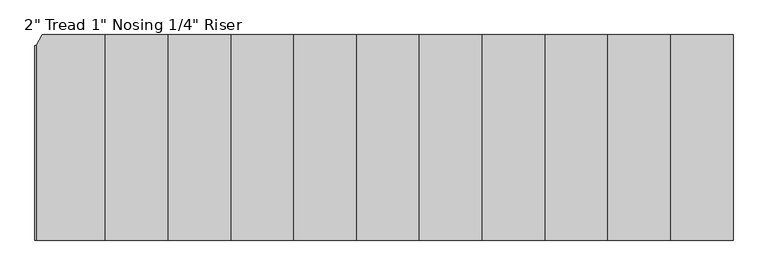
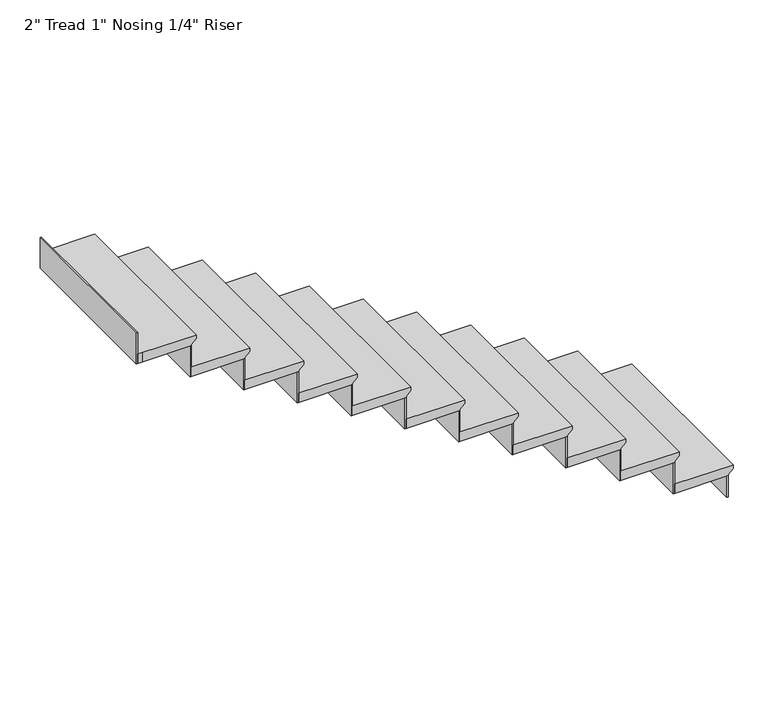
"""IFC4 building model written with IfcOpenShell, lengths in millimetres: stair flight geometry."""

from ifc_helpers import new_model, si_unit, origin, place, context, project, spatial, faceted_brep, source, transform, mapped, element, save


def stair_flight_13c2be00(model_context):
    return source(origin(), model_context, "Body", "Brep", [
        faceted_brep([(-10702.6822797, 5301.3500793, 150.2833333), (-10702.6822797, 5301.3500793, 169.3333333), (-10702.6822797, 4386.9500793, 169.3333333), (-10702.6822797, 4386.9500793, 150.2833333), (-10728.0822797, 5301.3500793, 124.8833333), (-10728.0822797, 4386.9500793, 124.8833333), (-11007.4822797, 5301.3500793, 169.3333333), (-11007.4822797, 4386.9500793, 169.3333333), (-10728.0822797, 4386.9500793, 118.5333333), (-11007.4822797, 4386.9500793, 118.5333333), (-11007.4822797, 5301.3500793, 118.5333333), (-10728.0822797, 5301.3500793, 118.5333333)], [[[0, 1, 2, 3]], [[4, 0, 3, 5]], [[2, 1, 6, 7]], [[8, 9, 10, 11]], [[2, 7, 9, 8, 5, 3]], [[8, 11, 4, 5]], [[6, 1, 0, 4, 11, 10]], [[7, 6, 10, 9]]]),
        faceted_brep([(-10728.0822797, 5301.3500793, 118.5333333), (-10728.0822797, 5301.3500793, 0.0), (-10734.4322797, 5301.3500793, 0.0), (-10734.4322797, 5301.3500793, 118.5333333), (-10728.0822797, 4386.9500793, 118.5333333), (-10734.4322797, 4386.9500793, 118.5333333), (-10734.4322797, 4386.9500793, 0.0), (-10728.0822797, 4386.9500793, 0.0)], [[[0, 1, 2, 3]], [[4, 5, 6, 7]], [[1, 0, 4, 7]], [[2, 1, 7, 6]], [[3, 2, 6, 5]], [[0, 3, 5, 4]]]),
        faceted_brep([(-11007.4822797, 5301.3500793, 287.8666667), (-11007.4822797, 5301.3500793, 118.5333333), (-11013.8322797, 5301.3500793, 118.5333333), (-11013.8322797, 5301.3500793, 287.8666667), (-11007.4822797, 4386.9500793, 287.8666667), (-11013.8322797, 4386.9500793, 287.8666667), (-11013.8322797, 4386.9500793, 118.5333333), (-11007.4822797, 4386.9500793, 118.5333333)], [[[0, 1, 2, 3]], [[4, 5, 6, 7]], [[1, 0, 4, 7]], [[2, 1, 7, 6]], [[3, 2, 6, 5]], [[0, 3, 5, 4]]]),
        faceted_brep([(-10982.0822797, 4386.9500793, 338.6666667), (-10982.0822797, 5301.3500793, 338.6666667), (-11286.8822797, 5301.3500793, 338.6666667), (-11286.8822797, 4386.9500793, 338.6666667), (-11007.4822797, 4386.9500793, 287.8666667), (-11286.8822797, 4386.9500793, 287.8666667), (-11286.8822797, 5301.3500793, 287.8666667), (-11007.4822797, 5301.3500793, 287.8666667), (-11007.4822797, 4386.9500793, 294.2166667), (-10982.0822797, 4386.9500793, 319.6166667), (-11007.4822797, 5301.3500793, 294.2166667), (-10982.0822797, 5301.3500793, 319.6166667)], [[[0, 1, 2, 3]], [[4, 5, 6, 7]], [[0, 3, 5, 4, 8, 9]], [[4, 7, 10, 8]], [[2, 1, 11, 10, 7, 6]], [[3, 2, 6, 5]], [[11, 1, 0, 9]], [[10, 11, 9, 8]]]),
        faceted_brep([(-11286.8822797, 5301.3500793, 457.2), (-11286.8822797, 5301.3500793, 287.8666667), (-11293.2322797, 5301.3500793, 287.8666667), (-11293.2322797, 5301.3500793, 457.2), (-11286.8822797, 4386.9500793, 457.2), (-11293.2322797, 4386.9500793, 457.2), (-11293.2322797, 4386.9500793, 287.8666667), (-11286.8822797, 4386.9500793, 287.8666667)], [[[0, 1, 2, 3]], [[4, 5, 6, 7]], [[1, 0, 4, 7]], [[2, 1, 7, 6]], [[3, 2, 6, 5]], [[0, 3, 5, 4]]]),
        faceted_brep([(-11261.4822797, 4386.9500793, 508.0), (-11261.4822797, 5301.3500793, 508.0), (-11566.2822797, 5301.3500793, 508.0), (-11566.2822797, 4386.9500793, 508.0), (-11286.8822797, 4386.9500793, 457.2), (-11566.2822797, 4386.9500793, 457.2), (-11566.2822797, 5301.3500793, 457.2), (-11286.8822797, 5301.3500793, 457.2), (-11286.8822797, 4386.9500793, 463.55), (-11261.4822797, 4386.9500793, 488.95), (-11286.8822797, 5301.3500793, 463.55), (-11261.4822797, 5301.3500793, 488.95)], [[[0, 1, 2, 3]], [[4, 5, 6, 7]], [[0, 3, 5, 4, 8, 9]], [[4, 7, 10, 8]], [[2, 1, 11, 10, 7, 6]], [[3, 2, 6, 5]], [[11, 1, 0, 9]], [[10, 11, 9, 8]]]),
        faceted_brep([(-11566.2822797, 5301.3500793, 626.5333333), (-11566.2822797, 5301.3500793, 457.2), (-11572.6322797, 5301.3500793, 457.2), (-11572.6322797, 5301.3500793, 626.5333333), (-11566.2822797, 4386.9500793, 626.5333333), (-11572.6322797, 4386.9500793, 626.5333333), (-11572.6322797, 4386.9500793, 457.2), (-11566.2822797, 4386.9500793, 457.2)], [[[0, 1, 2, 3]], [[4, 5, 6, 7]], [[1, 0, 4, 7]], [[2, 1, 7, 6]], [[3, 2, 6, 5]], [[0, 3, 5, 4]]]),
        faceted_brep([(-11540.8822797, 4386.9500793, 677.3333333), (-11540.8822797, 5301.3500793, 677.3333333), (-11845.6822797, 5301.3500793, 677.3333333), (-11845.6822797, 4386.9500793, 677.3333333), (-11566.2822797, 4386.9500793, 626.5333333), (-11845.6822797, 4386.9500793, 626.5333333), (-11845.6822797, 5301.3500793, 626.5333333), (-11566.2822797, 5301.3500793, 626.5333333), (-11566.2822797, 4386.9500793, 632.8833333), (-11540.8822797, 4386.9500793, 658.2833333), (-11566.2822797, 5301.3500793, 632.8833333), (-11540.8822797, 5301.3500793, 658.2833333)], [[[0, 1, 2, 3]], [[4, 5, 6, 7]], [[0, 3, 5, 4, 8, 9]], [[4, 7, 10, 8]], [[2, 1, 11, 10, 7, 6]], [[3, 2, 6, 5]], [[11, 1, 0, 9]], [[10, 11, 9, 8]]]),
        faceted_brep([(-11845.6822797, 5301.3500793, 795.8666667), (-11845.6822797, 5301.3500793, 626.5333333), (-11852.0322797, 5301.3500793, 626.5333333), (-11852.0322797, 5301.3500793, 795.8666667), (-11845.6822797, 4386.9500793, 795.8666667), (-11852.0322797, 4386.9500793, 795.8666667), (-11852.0322797, 4386.9500793, 626.5333333), (-11845.6822797, 4386.9500793, 626.5333333)], [[[0, 1, 2, 3]], [[4, 5, 6, 7]], [[1, 0, 4, 7]], [[2, 1, 7, 6]], [[3, 2, 6, 5]], [[0, 3, 5, 4]]]),
        faceted_brep([(-11820.2822797, 4386.9500793, 846.6666667), (-11820.2822797, 5301.3500793, 846.6666667), (-12125.0822797, 5301.3500793, 846.6666667), (-12125.0822797, 4386.9500793, 846.6666667), (-11845.6822797, 4386.9500793, 795.8666667), (-12125.0822797, 4386.9500793, 795.8666667), (-12125.0822797, 5301.3500793, 795.8666667), (-11845.6822797, 5301.3500793, 795.8666667), (-11845.6822797, 4386.9500793, 802.2166667), (-11820.2822797, 4386.9500793, 827.6166667), (-11845.6822797, 5301.3500793, 802.2166667), (-11820.2822797, 5301.3500793, 827.6166667)], [[[0, 1, 2, 3]], [[4, 5, 6, 7]], [[0, 3, 5, 4, 8, 9]], [[4, 7, 10, 8]], [[2, 1, 11, 10, 7, 6]], [[3, 2, 6, 5]], [[11, 1, 0, 9]], [[10, 11, 9, 8]]]),
        faceted_brep([(-12125.0822797, 5301.3500793, 965.2), (-12125.0822797, 5301.3500793, 795.8666667), (-12131.4322797, 5301.3500793, 795.8666667), (-12131.4322797, 5301.3500793, 965.2), (-12125.0822797, 4386.9500793, 965.2), (-12131.4322797, 4386.9500793, 965.2), (-12131.4322797, 4386.9500793, 795.8666667), (-12125.0822797, 4386.9500793, 795.8666667)], [[[0, 1, 2, 3]], [[4, 5, 6, 7]], [[1, 0, 4, 7]], [[2, 1, 7, 6]], [[3, 2, 6, 5]], [[0, 3, 5, 4]]]),
        faceted_brep([(-12099.6822797, 4386.9500793, 1016.0), (-12099.6822797, 5301.3500793, 1016.0), (-12404.4822797, 5301.3500793, 1016.0), (-12404.4822797, 4386.9500793, 1016.0), (-12125.0822797, 4386.9500793, 965.2), (-12404.4822797, 4386.9500793, 965.2), (-12404.4822797, 5301.3500793, 965.2), (-12125.0822797, 5301.3500793, 965.2), (-12125.0822797, 4386.9500793, 971.55), (-12099.6822797, 4386.9500793, 996.95), (-12125.0822797, 5301.3500793, 971.55), (-12099.6822797, 5301.3500793, 996.95)], [[[0, 1, 2, 3]], [[4, 5, 6, 7]], [[0, 3, 5, 4, 8, 9]], [[4, 7, 10, 8]], [[2, 1, 11, 10, 7, 6]], [[3, 2, 6, 5]], [[11, 1, 0, 9]], [[10, 11, 9, 8]]]),
        faceted_brep([(-12404.4822797, 5301.3500793, 1134.5333333), (-12404.4822797, 5301.3500793, 965.2), (-12410.8322797, 5301.3500793, 965.2), (-12410.8322797, 5301.3500793, 1134.5333333), (-12404.4822797, 4386.9500793, 1134.5333333), (-12410.8322797, 4386.9500793, 1134.5333333), (-12410.8322797, 4386.9500793, 965.2), (-12404.4822797, 4386.9500793, 965.2)], [[[0, 1, 2, 3]], [[4, 5, 6, 7]], [[1, 0, 4, 7]], [[2, 1, 7, 6]], [[3, 2, 6, 5]], [[0, 3, 5, 4]]]),
        faceted_brep([(-12379.0822797, 4386.9500793, 1185.3333333), (-12379.0822797, 5301.3500793, 1185.3333333), (-12683.8822797, 5301.3500793, 1185.3333333), (-12683.8822797, 4386.9500793, 1185.3333333), (-12404.4822797, 4386.9500793, 1134.5333333), (-12683.8822797, 4386.9500793, 1134.5333333), (-12683.8822797, 5301.3500793, 1134.5333333), (-12404.4822797, 5301.3500793, 1134.5333333), (-12404.4822797, 4386.9500793, 1140.8833333), (-12379.0822797, 4386.9500793, 1166.2833333), (-12404.4822797, 5301.3500793, 1140.8833333), (-12379.0822797, 5301.3500793, 1166.2833333)], [[[0, 1, 2, 3]], [[4, 5, 6, 7]], [[0, 3, 5, 4, 8, 9]], [[4, 7, 10, 8]], [[2, 1, 11, 10, 7, 6]], [[3, 2, 6, 5]], [[11, 1, 0, 9]], [[10, 11, 9, 8]]]),
        faceted_brep([(-12683.8822797, 5301.3500793, 1303.8666667), (-12683.8822797, 5301.3500793, 1134.5333333), (-12690.2322797, 5301.3500793, 1134.5333333), (-12690.2322797, 5301.3500793, 1303.8666667), (-12683.8822797, 4386.9500793, 1303.8666667), (-12690.2322797, 4386.9500793, 1303.8666667), (-12690.2322797, 4386.9500793, 1134.5333333), (-12683.8822797, 4386.9500793, 1134.5333333)], [[[0, 1, 2, 3]], [[4, 5, 6, 7]], [[1, 0, 4, 7]], [[2, 1, 7, 6]], [[3, 2, 6, 5]], [[0, 3, 5, 4]]]),
        faceted_brep([(-12658.4822797, 4386.9500793, 1354.6666667), (-12658.4822797, 5301.3500793, 1354.6666667), (-12963.2822797, 5301.3500793, 1354.6666667), (-12963.2822797, 4386.9500793, 1354.6666667), (-12683.8822797, 4386.9500793, 1303.8666667), (-12963.2822797, 4386.9500793, 1303.8666667), (-12963.2822797, 5301.3500793, 1303.8666667), (-12683.8822797, 5301.3500793, 1303.8666667), (-12683.8822797, 4386.9500793, 1310.2166667), (-12658.4822797, 4386.9500793, 1335.6166667), (-12683.8822797, 5301.3500793, 1310.2166667), (-12658.4822797, 5301.3500793, 1335.6166667)], [[[0, 1, 2, 3]], [[4, 5, 6, 7]], [[0, 3, 5, 4, 8, 9]], [[4, 7, 10, 8]], [[2, 1, 11, 10, 7, 6]], [[3, 2, 6, 5]], [[11, 1, 0, 9]], [[10, 11, 9, 8]]]),
        faceted_brep([(-12963.2822797, 5301.3500793, 1473.2), (-12963.2822797, 5301.3500793, 1303.8666667), (-12969.6322797, 5301.3500793, 1303.8666667), (-12969.6322797, 5301.3500793, 1473.2), (-12963.2822797, 4386.9500793, 1473.2), (-12969.6322797, 4386.9500793, 1473.2), (-12969.6322797, 4386.9500793, 1303.8666667), (-12963.2822797, 4386.9500793, 1303.8666667)], [[[0, 1, 2, 3]], [[4, 5, 6, 7]], [[1, 0, 4, 7]], [[2, 1, 7, 6]], [[3, 2, 6, 5]], [[0, 3, 5, 4]]]),
        faceted_brep([(-12937.8822797, 4386.9500793, 1524.0), (-12937.8822797, 5301.3500793, 1524.0), (-13242.6822797, 5301.3500793, 1524.0), (-13242.6822797, 4386.9500793, 1524.0), (-12963.2822797, 4386.9500793, 1473.2), (-13242.6822797, 4386.9500793, 1473.2), (-13242.6822797, 5301.3500793, 1473.2), (-12963.2822797, 5301.3500793, 1473.2), (-12963.2822797, 4386.9500793, 1479.55), (-12937.8822797, 4386.9500793, 1504.95), (-12963.2822797, 5301.3500793, 1479.55), (-12937.8822797, 5301.3500793, 1504.95)], [[[0, 1, 2, 3]], [[4, 5, 6, 7]], [[0, 3, 5, 4, 8, 9]], [[4, 7, 10, 8]], [[2, 1, 11, 10, 7, 6]], [[3, 2, 6, 5]], [[11, 1, 0, 9]], [[10, 11, 9, 8]]]),
        faceted_brep([(-13242.6822797, 5301.3500793, 1642.5333333), (-13242.6822797, 5301.3500793, 1473.2), (-13249.0322797, 5301.3500793, 1473.2), (-13249.0322797, 5301.3500793, 1642.5333333), (-13242.6822797, 4386.9500793, 1642.5333333), (-13249.0322797, 4386.9500793, 1642.5333333), (-13249.0322797, 4386.9500793, 1473.2), (-13242.6822797, 4386.9500793, 1473.2)], [[[0, 1, 2, 3]], [[4, 5, 6, 7]], [[1, 0, 4, 7]], [[2, 1, 7, 6]], [[3, 2, 6, 5]], [[0, 3, 5, 4]]]),
        faceted_brep([(-13217.2822797, 4386.9500793, 1693.3333333), (-13217.2822797, 5301.3500793, 1693.3333333), (-13522.0822797, 5301.3500793, 1693.3333333), (-13522.0822797, 4386.9500793, 1693.3333333), (-13242.6822797, 4386.9500793, 1642.5333333), (-13522.0822797, 4386.9500793, 1642.5333333), (-13522.0822797, 5301.3500793, 1642.5333333), (-13242.6822797, 5301.3500793, 1642.5333333), (-13242.6822797, 4386.9500793, 1648.8833333), (-13217.2822797, 4386.9500793, 1674.2833333), (-13242.6822797, 5301.3500793, 1648.8833333), (-13217.2822797, 5301.3500793, 1674.2833333)], [[[0, 1, 2, 3]], [[4, 5, 6, 7]], [[0, 3, 5, 4, 8, 9]], [[4, 7, 10, 8]], [[2, 1, 11, 10, 7, 6]], [[3, 2, 6, 5]], [[11, 1, 0, 9]], [[10, 11, 9, 8]]]),
        faceted_brep([(-13801.4822797, 5254.1625376, 1981.2), (-13801.4822797, 5254.1625376, 1811.8666667), (-13807.8322797, 5254.1625376, 1811.8666667), (-13807.8322797, 5254.1625376, 1981.2), (-13801.4822797, 4386.9500793, 1981.2), (-13807.8322797, 4386.9500793, 1981.2), (-13807.8322797, 4386.9500793, 1811.8666667), (-13801.4822797, 4386.9500793, 1811.8666667)], [[[0, 1, 2, 3]], [[4, 5, 6, 7]], [[1, 0, 4, 7]], [[2, 1, 7, 6]], [[3, 2, 6, 5]], [[0, 3, 5, 4]]]),
        faceted_brep([(-13522.0822797, 5301.3500793, 1811.8666667), (-13522.0822797, 5301.3500793, 1642.5333333), (-13528.4322797, 5301.3500793, 1642.5333333), (-13528.4322797, 5301.3500793, 1811.8666667), (-13522.0822797, 4386.9500793, 1811.8666667), (-13528.4322797, 4386.9500793, 1811.8666667), (-13528.4322797, 4386.9500793, 1642.5333333), (-13522.0822797, 4386.9500793, 1642.5333333)], [[[0, 1, 2, 3]], [[4, 5, 6, 7]], [[1, 0, 4, 7]], [[2, 1, 7, 6]], [[3, 2, 6, 5]], [[0, 3, 5, 4]]]),
        faceted_brep([(-13801.4822797, 4386.9500793, 1862.6666667), (-13776.0822797, 4386.9500793, 1862.6666667), (-13496.6822797, 4386.9500793, 1862.6666667), (-13496.6822797, 5301.3500793, 1862.6666667), (-13776.0822797, 5301.3500793, 1862.6666667), (-13801.4822797, 5254.1625376, 1862.6666667), (-13776.0822797, 4386.9500793, 1811.8666667), (-13801.4822797, 4386.9500793, 1811.8666667), (-13801.4822797, 5254.1625376, 1811.8666667), (-13776.0822797, 5301.3500793, 1811.8666667), (-13522.0822797, 5301.3500793, 1811.8666667), (-13522.0822797, 4386.9500793, 1811.8666667), (-13522.0822797, 4386.9500793, 1818.2166667), (-13496.6822797, 4386.9500793, 1843.6166667), (-13522.0822797, 5301.3500793, 1818.2166667), (-13496.6822797, 5301.3500793, 1843.6166667)], [[[0, 1, 2, 3, 4, 5]], [[6, 7, 8, 9, 10, 11]], [[1, 0, 7, 6]], [[2, 1, 6, 11, 12, 13]], [[11, 10, 14, 12]], [[4, 3, 15, 14, 10, 9]], [[5, 4, 9, 8]], [[0, 5, 8, 7]], [[15, 3, 2, 13]], [[14, 15, 13, 12]]]),
    ])


if __name__ == "__main__":
    model = new_model("IFC4")
    model_context = context("Model", 3, world=origin())
    ifc_project = project(units=[si_unit("LENGTHUNIT", "METRE", prefix="MILLI")], contexts=[model_context])
    site = spatial("IfcSite", under=ifc_project)
    building = spatial("IfcBuilding", under=site)
    placement = place(None, origin())
    stair_flight_shape = stair_flight_13c2be00(model_context)
    element("IfcStairFlight", 1, ObjectType="2\" Tread 1\" Nosing 1/4\" Riser", at=placement, inside=building, context=model_context, shape_type="MappedRepresentation", body=[
        mapped(stair_flight_shape, transform((0.0, 0.0, 0.0), x_axis=(1.0, 0.0, 0.0), y_axis=(0.0, 1.0, 0.0), z_axis=(0.0, 0.0, 1.0))),
    ])
    save(model, "model.ifc")
